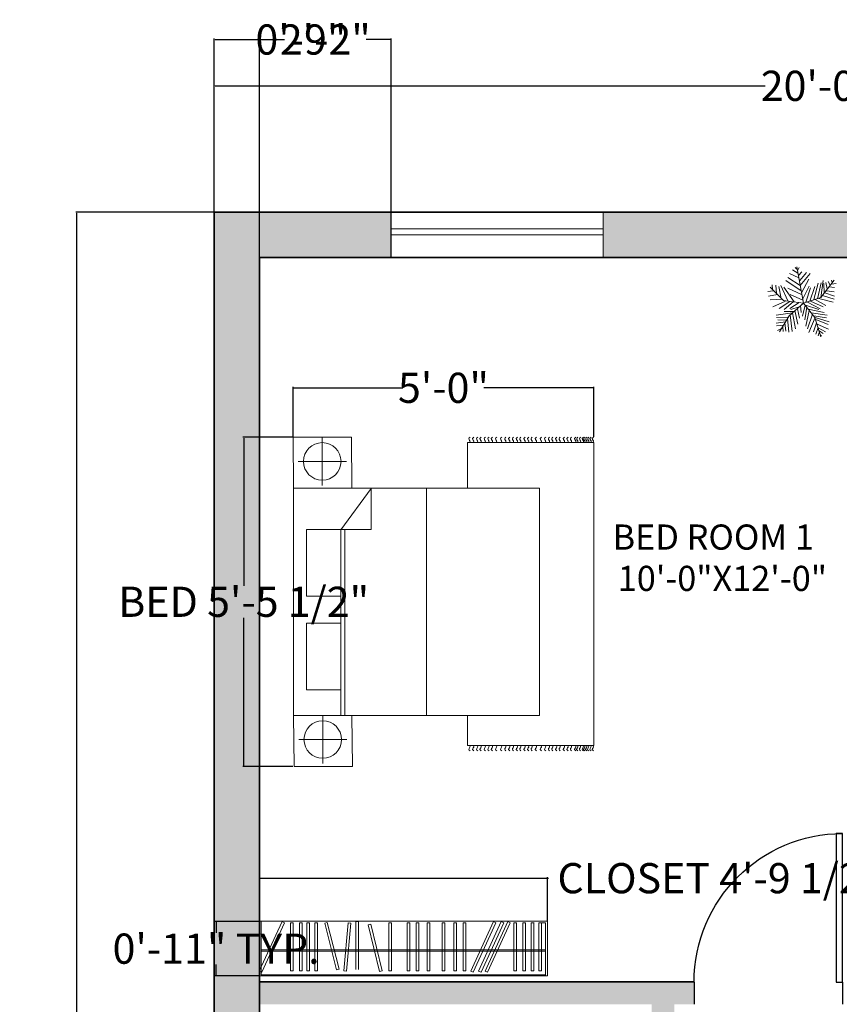
# Model space of a CAD drawing. Units: inches. Extents: x 143233372 to 143233714, y 112671713 to 112672292.
# Tile 6 of 7: x 143233378 to 143233541, y 112672092 to 112672287. Entities that reach past the tile are written whole.
import ezdxf

# ---------------------------------------------------------------- set-up
doc = ezdxf.new("R2010")
doc.units = ezdxf.units.IN
doc.header["$MEASUREMENT"] = 0
doc.layers.get('0').update_dxf_attribs({"color": 104})
for name, color, linetype, lineweight in [('A-ANNO-DIMS', 2, 'Continuous', 18), ('A-AREA-IDEN', 7, 'Continuous', 18), ('closet', 23, 'Continuous', 18), ('doors', 32, 'Continuous', 25), ('furniture', 23, 'Continuous', 18), ('L-PLNT', 92, 'Continuous', 13), ('walls', 7, 'Continuous', 35), ('windows', 4, 'Continuous', 18)]:
    doc.layers.add(name, color=color, linetype=linetype, lineweight=lineweight)
doc.layers.add('A-WALL-PATT', color=18, linetype='Continuous', lineweight=9, true_color=0x000000)
doc.styles.get("Standard").update_dxf_attribs({"font": 'arial.ttf'})
doc.dimstyles.get("Standard").update_dxf_attribs({"dimtxt": 6, "dimasz": 0.18, "dimexe": 0.18, "dimexo": 0.0625, "dimgap": 0.09, "dimtad": 0, "dimtih": 1, "dimtoh": 1, "dimzin": 0, "dimdsep": 46, "dimlunit": 3, "dimtxsty": 'Standard', "dimcen": 0.09, "dimadec": 0, "dimazin": 0, "dimtfac": 1, "dimtofl": 0, "dimtmove": 0, "dimatfit": 3, "dimfxl": 1, "dimtolj": 1, "dimtzin": 0, "dimarcsym": 0})

# ---------------------------------------------------------------- blocks, each defined once
blk = doc.blocks.new('CARPET')
at = {"layer": 'furniture'}
for p, q in [((-51.53, -98.11), (-51.53, -55.12)), ((-51.53, -55.12), (-41.27, -55.12)), ((36, -55.12), (51.55, -55.12)), ((51.55, -55.12), (51.55, -98.11)), ((51.55, -98.11), (-51.53, -98.11))]:
    blk.add_line(p, q, dxfattribs=at)
for points, knots in [([(-53.37, -55.99), (-53.22, -55.8), (-52.9, -55.41), (-52.34, -55.8), (-51.89, -56.08), (-51.65, -55.91), (-51.53, -55.83)], [0, 0, 0, 0, 0.653278, 1.290138, 1.740457, 2.114451, 2.114451, 2.114451, 2.114451]), ([(-53.37, -57.26), (-53.22, -57.07), (-52.9, -56.67), (-52.34, -57.07), (-51.89, -57.35), (-51.65, -57.17), (-51.53, -57.1)], [0, 0, 0, 0, 0.653278, 1.290138, 1.740457, 2.114451, 2.114451, 2.114451, 2.114451]), ([(53.37, -55.99), (53.22, -55.8), (52.9, -55.41), (52.34, -55.8), (51.89, -56.08), (51.65, -55.91), (51.53, -55.83)], [0, 0, 0, 0, 0.653278, 1.290138, 1.740457, 2.114451, 2.114451, 2.114451, 2.114451]), ([(53.37, -57.26), (53.22, -57.07), (52.9, -56.67), (52.34, -57.07), (51.89, -57.35), (51.65, -57.17), (51.53, -57.1)], [0, 0, 0, 0, 0.653278, 1.290138, 1.740457, 2.114451, 2.114451, 2.114451, 2.114451]), ([(-53.37, -58.59), (-53.22, -58.4), (-52.9, -58.01), (-52.34, -58.4), (-51.89, -58.68), (-51.65, -58.5), (-51.53, -58.43)], [0, 0, 0, 0, 0.653278, 1.290138, 1.740457, 2.114451, 2.114451, 2.114451, 2.114451]), ([(-53.37, -59.78), (-53.22, -59.58), (-52.9, -59.19), (-52.34, -59.58), (-51.89, -59.86), (-51.65, -59.69), (-51.53, -59.61)], [0, 0, 0, 0, 0.653278, 1.290138, 1.740457, 2.114451, 2.114451, 2.114451, 2.114451]), ([(53.37, -58.59), (53.22, -58.4), (52.9, -58.01), (52.34, -58.4), (51.89, -58.68), (51.65, -58.5), (51.53, -58.43)], [0, 0, 0, 0, 0.653278, 1.290138, 1.740457, 2.114451, 2.114451, 2.114451, 2.114451]), ([(53.37, -59.78), (53.22, -59.58), (52.9, -59.19), (52.34, -59.58), (51.89, -59.86), (51.65, -59.69), (51.53, -59.61)], [0, 0, 0, 0, 0.653278, 1.290138, 1.740457, 2.114451, 2.114451, 2.114451, 2.114451]), ([(-53.37, -61.22), (-53.22, -61.02), (-52.9, -60.63), (-52.34, -61.02), (-51.89, -61.3), (-51.65, -61.13), (-51.53, -61.05)], [0, 0, 0, 0, 0.653278, 1.290138, 1.740457, 2.114451, 2.114451, 2.114451, 2.114451]), ([(-53.37, -62.44), (-53.22, -62.25), (-52.9, -61.86), (-52.34, -62.25), (-51.89, -62.53), (-51.65, -62.36), (-51.53, -62.28)], [0, 0, 0, 0, 0.653278, 1.290138, 1.740457, 2.114451, 2.114451, 2.114451, 2.114451]), ([(-53.37, -63.63), (-53.22, -63.43), (-52.9, -63.04), (-52.34, -63.43), (-51.89, -63.72), (-51.65, -63.54), (-51.53, -63.46)], [0, 0, 0, 0, 0.653278, 1.290138, 1.740457, 2.114451, 2.114451, 2.114451, 2.114451]), ([(53.37, -61.22), (53.22, -61.02), (52.9, -60.63), (52.34, -61.02), (51.89, -61.3), (51.65, -61.13), (51.53, -61.05)], [0, 0, 0, 0, 0.653278, 1.290138, 1.740457, 2.114451, 2.114451, 2.114451, 2.114451]), ([(53.37, -62.44), (53.22, -62.25), (52.9, -61.86), (52.34, -62.25), (51.89, -62.53), (51.65, -62.36), (51.53, -62.28)], [0, 0, 0, 0, 0.653278, 1.290138, 1.740457, 2.114451, 2.114451, 2.114451, 2.114451]), ([(53.37, -63.63), (53.22, -63.43), (52.9, -63.04), (52.34, -63.43), (51.89, -63.72), (51.65, -63.54), (51.53, -63.46)], [0, 0, 0, 0, 0.653278, 1.290138, 1.740457, 2.114451, 2.114451, 2.114451, 2.114451]), ([(-53.37, -65.07), (-53.22, -64.87), (-52.9, -64.48), (-52.34, -64.87), (-51.89, -65.15), (-51.65, -64.98), (-51.53, -64.9)], [0, 0, 0, 0, 0.653278, 1.290138, 1.740457, 2.114451, 2.114451, 2.114451, 2.114451]), ([(-53.37, -66.76), (-53.22, -66.56), (-52.9, -66.17), (-52.34, -66.56), (-51.89, -66.84), (-51.65, -66.67), (-51.53, -66.59)], [0, 0, 0, 0, 0.653278, 1.290138, 1.740457, 2.114451, 2.114451, 2.114451, 2.114451]), ([(53.37, -65.07), (53.22, -64.87), (52.9, -64.48), (52.34, -64.87), (51.89, -65.15), (51.65, -64.98), (51.53, -64.9)], [0, 0, 0, 0, 0.653278, 1.290138, 1.740457, 2.114451, 2.114451, 2.114451, 2.114451]), ([(53.37, -66.76), (53.22, -66.56), (52.9, -66.17), (52.34, -66.56), (51.89, -66.84), (51.65, -66.67), (51.53, -66.59)], [0, 0, 0, 0, 0.653278, 1.290138, 1.740457, 2.114451, 2.114451, 2.114451, 2.114451]), ([(-53.37, -68.2), (-53.22, -68), (-52.9, -67.61), (-52.34, -68), (-51.89, -68.28), (-51.65, -68.11), (-51.53, -68.03)], [0, 0, 0, 0, 0.653278, 1.290138, 1.740457, 2.114451, 2.114451, 2.114451, 2.114451]), ([(-53.37, -69.53), (-53.22, -69.33), (-52.9, -68.94), (-52.34, -69.33), (-51.89, -69.61), (-51.65, -69.44), (-51.53, -69.36)], [0, 0, 0, 0, 0.653278, 1.290138, 1.740457, 2.114451, 2.114451, 2.114451, 2.114451]), ([(-53.37, -70.79), (-53.22, -70.6), (-52.9, -70.21), (-52.34, -70.6), (-51.89, -70.88), (-51.65, -70.7), (-51.53, -70.63)], [0, 0, 0, 0, 0.653278, 1.290138, 1.740457, 2.114451, 2.114451, 2.114451, 2.114451]), ([(53.37, -68.2), (53.22, -68), (52.9, -67.61), (52.34, -68), (51.89, -68.28), (51.65, -68.11), (51.53, -68.03)], [0, 0, 0, 0, 0.653278, 1.290138, 1.740457, 2.114451, 2.114451, 2.114451, 2.114451]), ([(53.37, -69.53), (53.22, -69.33), (52.9, -68.94), (52.34, -69.33), (51.89, -69.61), (51.65, -69.44), (51.53, -69.36)], [0, 0, 0, 0, 0.653278, 1.290138, 1.740457, 2.114451, 2.114451, 2.114451, 2.114451]), ([(53.37, -70.79), (53.22, -70.6), (52.9, -70.21), (52.34, -70.6), (51.89, -70.88), (51.65, -70.7), (51.53, -70.63)], [0, 0, 0, 0, 0.653278, 1.290138, 1.740457, 2.114451, 2.114451, 2.114451, 2.114451]), ([(-53.37, -72.12), (-53.22, -71.93), (-52.9, -71.54), (-52.34, -71.93), (-51.89, -72.21), (-51.65, -72.04), (-51.53, -71.96)], [0, 0, 0, 0, 0.653278, 1.290138, 1.740457, 2.114451, 2.114451, 2.114451, 2.114451]), ([(-53.37, -73.31), (-53.22, -73.11), (-52.9, -72.72), (-52.34, -73.11), (-51.89, -73.4), (-51.65, -73.22), (-51.53, -73.14)], [0, 0, 0, 0, 0.653278, 1.290138, 1.740457, 2.114451, 2.114451, 2.114451, 2.114451]), ([(53.37, -72.12), (53.22, -71.93), (52.9, -71.54), (52.34, -71.93), (51.89, -72.21), (51.65, -72.04), (51.53, -71.96)], [0, 0, 0, 0, 0.653278, 1.290138, 1.740457, 2.114451, 2.114451, 2.114451, 2.114451]), ([(53.37, -73.31), (53.22, -73.11), (52.9, -72.72), (52.34, -73.11), (51.89, -73.4), (51.65, -73.22), (51.53, -73.14)], [0, 0, 0, 0, 0.653278, 1.290138, 1.740457, 2.114451, 2.114451, 2.114451, 2.114451]), ([(-53.37, -74.75), (-53.22, -74.55), (-52.9, -74.16), (-52.34, -74.55), (-51.89, -74.83), (-51.65, -74.66), (-51.53, -74.58)], [0, 0, 0, 0, 0.653278, 1.290138, 1.740457, 2.114451, 2.114451, 2.114451, 2.114451]), ([(-53.37, -75.98), (-53.22, -75.78), (-52.9, -75.39), (-52.34, -75.78), (-51.89, -76.06), (-51.65, -75.89), (-51.53, -75.81)], [0, 0, 0, 0, 0.653278, 1.290138, 1.740457, 2.114451, 2.114451, 2.114451, 2.114451]), ([(-53.37, -77.16), (-53.22, -76.96), (-52.9, -76.57), (-52.34, -76.96), (-51.89, -77.25), (-51.65, -77.07), (-51.53, -76.99)], [0, 0, 0, 0, 0.653278, 1.290138, 1.740457, 2.114451, 2.114451, 2.114451, 2.114451]), ([(53.37, -74.75), (53.22, -74.55), (52.9, -74.16), (52.34, -74.55), (51.89, -74.83), (51.65, -74.66), (51.53, -74.58)], [0, 0, 0, 0, 0.653278, 1.290138, 1.740457, 2.114451, 2.114451, 2.114451, 2.114451]), ([(53.37, -75.98), (53.22, -75.78), (52.9, -75.39), (52.34, -75.78), (51.89, -76.06), (51.65, -75.89), (51.53, -75.81)], [0, 0, 0, 0, 0.653278, 1.290138, 1.740457, 2.114451, 2.114451, 2.114451, 2.114451]), ([(53.37, -77.16), (53.22, -76.96), (52.9, -76.57), (52.34, -76.96), (51.89, -77.25), (51.65, -77.07), (51.53, -76.99)], [0, 0, 0, 0, 0.653278, 1.290138, 1.740457, 2.114451, 2.114451, 2.114451, 2.114451]), ([(-53.37, -78.6), (-53.22, -78.4), (-52.9, -78.01), (-52.34, -78.4), (-51.89, -78.68), (-51.65, -78.51), (-51.53, -78.43)], [0, 0, 0, 0, 0.653278, 1.290138, 1.740457, 2.114451, 2.114451, 2.114451, 2.114451]), ([(-53.37, -80.29), (-53.22, -80.09), (-52.9, -79.7), (-52.34, -80.09), (-51.89, -80.37), (-51.65, -80.2), (-51.53, -80.12)], [0, 0, 0, 0, 0.653278, 1.290138, 1.740457, 2.114451, 2.114451, 2.114451, 2.114451]), ([(53.37, -78.6), (53.22, -78.4), (52.9, -78.01), (52.34, -78.4), (51.89, -78.68), (51.65, -78.51), (51.53, -78.43)], [0, 0, 0, 0, 0.653278, 1.290138, 1.740457, 2.114451, 2.114451, 2.114451, 2.114451]), ([(53.37, -80.29), (53.22, -80.09), (52.9, -79.7), (52.34, -80.09), (51.89, -80.37), (51.65, -80.2), (51.53, -80.12)], [0, 0, 0, 0, 0.653278, 1.290138, 1.740457, 2.114451, 2.114451, 2.114451, 2.114451]), ([(-53.37, -81.73), (-53.22, -81.53), (-52.9, -81.14), (-52.34, -81.53), (-51.89, -81.81), (-51.65, -81.64), (-51.53, -81.56)], [0, 0, 0, 0, 0.653278, 1.290138, 1.740457, 2.114451, 2.114451, 2.114451, 2.114451]), ([(-53.37, -83.06), (-53.22, -82.86), (-52.9, -82.47), (-52.34, -82.86), (-51.89, -83.14), (-51.65, -82.97), (-51.53, -82.89)], [0, 0, 0, 0, 0.653278, 1.290138, 1.740457, 2.114451, 2.114451, 2.114451, 2.114451]), ([(-53.37, -84.18), (-53.22, -83.99), (-52.9, -83.6), (-52.34, -83.99), (-51.89, -84.27), (-51.65, -84.09), (-51.53, -84.02)], [0, 0, 0, 0, 0.653278, 1.290138, 1.740457, 2.114451, 2.114451, 2.114451, 2.114451]), ([(53.37, -81.73), (53.22, -81.53), (52.9, -81.14), (52.34, -81.53), (51.89, -81.81), (51.65, -81.64), (51.53, -81.56)], [0, 0, 0, 0, 0.653278, 1.290138, 1.740457, 2.114451, 2.114451, 2.114451, 2.114451]), ([(53.37, -83.06), (53.22, -82.86), (52.9, -82.47), (52.34, -82.86), (51.89, -83.14), (51.65, -82.97), (51.53, -82.89)], [0, 0, 0, 0, 0.653278, 1.290138, 1.740457, 2.114451, 2.114451, 2.114451, 2.114451]), ([(53.37, -84.18), (53.22, -83.99), (52.9, -83.6), (52.34, -83.99), (51.89, -84.27), (51.65, -84.09), (51.53, -84.02)], [0, 0, 0, 0, 0.653278, 1.290138, 1.740457, 2.114451, 2.114451, 2.114451, 2.114451]), ([(-53.37, -85.51), (-53.22, -85.32), (-52.9, -84.93), (-52.34, -85.32), (-51.89, -85.6), (-51.65, -85.42), (-51.53, -85.35)], [0, 0, 0, 0, 0.653278, 1.290138, 1.740457, 2.114451, 2.114451, 2.114451, 2.114451]), ([(-53.37, -86.7), (-53.22, -86.5), (-52.9, -86.11), (-52.34, -86.5), (-51.89, -86.78), (-51.65, -86.61), (-51.53, -86.53)], [0, 0, 0, 0, 0.653278, 1.290138, 1.740457, 2.114451, 2.114451, 2.114451, 2.114451]), ([(53.37, -85.51), (53.22, -85.32), (52.9, -84.93), (52.34, -85.32), (51.89, -85.6), (51.65, -85.42), (51.53, -85.35)], [0, 0, 0, 0, 0.653278, 1.290138, 1.740457, 2.114451, 2.114451, 2.114451, 2.114451]), ([(53.37, -86.7), (53.22, -86.5), (52.9, -86.11), (52.34, -86.5), (51.89, -86.78), (51.65, -86.61), (51.53, -86.53)], [0, 0, 0, 0, 0.653278, 1.290138, 1.740457, 2.114451, 2.114451, 2.114451, 2.114451]), ([(-53.37, -88.14), (-53.22, -87.94), (-52.9, -87.55), (-52.34, -87.94), (-51.89, -88.22), (-51.65, -88.05), (-51.53, -87.97)], [0, 0, 0, 0, 0.653278, 1.290138, 1.740457, 2.114451, 2.114451, 2.114451, 2.114451]), ([(-53.37, -89.36), (-53.22, -89.17), (-52.9, -88.78), (-52.34, -89.17), (-51.89, -89.45), (-51.65, -89.28), (-51.53, -89.2)], [0, 0, 0, 0, 0.653278, 1.290138, 1.740457, 2.114451, 2.114451, 2.114451, 2.114451]), ([(-53.37, -90.55), (-53.22, -90.35), (-52.9, -89.96), (-52.34, -90.35), (-51.89, -90.64), (-51.65, -90.46), (-51.53, -90.38)], [0, 0, 0, 0, 0.653278, 1.290138, 1.740457, 2.114451, 2.114451, 2.114451, 2.114451]), ([(53.37, -88.14), (53.22, -87.94), (52.9, -87.55), (52.34, -87.94), (51.89, -88.22), (51.65, -88.05), (51.53, -87.97)], [0, 0, 0, 0, 0.653278, 1.290138, 1.740457, 2.114451, 2.114451, 2.114451, 2.114451]), ([(53.37, -89.36), (53.22, -89.17), (52.9, -88.78), (52.34, -89.17), (51.89, -89.45), (51.65, -89.28), (51.53, -89.2)], [0, 0, 0, 0, 0.653278, 1.290138, 1.740457, 2.114451, 2.114451, 2.114451, 2.114451]), ([(53.37, -90.55), (53.22, -90.35), (52.9, -89.96), (52.34, -90.35), (51.9, -90.63), (51.66, -90.47), (51.55, -90.4)], [0, 0, 0, 0, 0.653278, 1.290138, 1.740457, 2.0926, 2.0926, 2.0926, 2.0926]), ([(-53.37, -91.99), (-53.22, -91.79), (-52.9, -91.4), (-52.34, -91.79), (-51.89, -92.07), (-51.65, -91.9), (-51.53, -91.82)], [0, 0, 0, 0, 0.653278, 1.290138, 1.740457, 2.114451, 2.114451, 2.114451, 2.114451]), ([(-53.37, -92.69), (-53.22, -92.48), (-52.9, -92.08), (-52.35, -92.49), (-51.89, -92.77), (-51.65, -92.6), (-51.53, -92.52)], [0, 0, 0, 0, 0.663904, 1.307406, 1.757725, 2.131719, 2.131719, 2.131719, 2.131719]), ([(-53.37, -93.61), (-53.22, -93.42), (-52.9, -93.03), (-52.34, -93.42), (-51.89, -93.7), (-51.65, -93.52), (-51.53, -93.45)], [0, 0, 0, 0, 0.653278, 1.290138, 1.740457, 2.114451, 2.114451, 2.114451, 2.114451]), ([(53.37, -91.99), (53.22, -91.79), (52.9, -91.4), (52.34, -91.79), (51.9, -92.07), (51.66, -91.91), (51.55, -91.83)], [0, 0, 0, 0, 0.653278, 1.290138, 1.740457, 2.0926, 2.0926, 2.0926, 2.0926]), ([(53.37, -92.69), (53.22, -92.49), (52.9, -92.09), (52.34, -92.49), (51.9, -92.77), (51.66, -92.61), (51.55, -92.53)], [0, 0, 0, 0, 0.656792, 1.295826, 1.746145, 2.098292, 2.098292, 2.098292, 2.098292]), ([(53.37, -93.66), (53.22, -93.46), (52.9, -93.07), (52.34, -93.46), (51.9, -93.74), (51.66, -93.58), (51.55, -93.5)], [0, 0, 0, 0, 0.653278, 1.290138, 1.740457, 2.0926, 2.0926, 2.0926, 2.0926]), ([(-53.37, -94.55), (-53.22, -94.35), (-52.9, -93.96), (-52.34, -94.35), (-51.89, -94.63), (-51.65, -94.46), (-51.53, -94.38)], [0, 0, 0, 0, 0.653278, 1.290138, 1.740457, 2.114451, 2.114451, 2.114451, 2.114451]), ([(-53.37, -95.05), (-53.22, -94.85), (-52.9, -94.46), (-52.34, -94.85), (-51.89, -95.14), (-51.65, -94.96), (-51.53, -94.88)], [0, 0, 0, 0, 0.653278, 1.290138, 1.740457, 2.114451, 2.114451, 2.114451, 2.114451]), ([(-53.37, -95.73), (-53.22, -95.54), (-52.9, -95.15), (-52.34, -95.54), (-51.89, -95.82), (-51.65, -95.65), (-51.53, -95.57)], [0, 0, 0, 0, 0.653278, 1.290138, 1.740457, 2.114451, 2.114451, 2.114451, 2.114451]), ([(-53.37, -96.38), (-53.22, -96.18), (-52.9, -95.79), (-52.34, -96.18), (-51.89, -96.47), (-51.65, -96.29), (-51.53, -96.21)], [0, 0, 0, 0, 0.653278, 1.290138, 1.740457, 2.114451, 2.114451, 2.114451, 2.114451]), ([(-53.37, -97.17), (-53.22, -96.98), (-52.9, -96.59), (-52.34, -96.98), (-51.89, -97.26), (-51.65, -97.08), (-51.53, -97.01)], [0, 0, 0, 0, 0.653278, 1.290138, 1.740457, 2.114451, 2.114451, 2.114451, 2.114451]), ([(53.37, -95.78), (53.22, -95.58), (52.9, -95.19), (52.34, -95.58), (51.89, -95.86), (51.65, -95.69), (51.53, -95.61)], [0, 0, 0, 0, 0.653278, 1.290138, 1.740457, 2.114451, 2.114451, 2.114451, 2.114451]), ([(53.37, -96.43), (53.22, -96.23), (52.9, -95.84), (52.34, -96.23), (51.89, -96.51), (51.65, -96.34), (51.53, -96.26)], [0, 0, 0, 0, 0.653278, 1.290138, 1.740457, 2.114451, 2.114451, 2.114451, 2.114451]), ([(53.37, -97.22), (53.22, -97.02), (52.9, -96.63), (52.34, -97.02), (51.89, -97.3), (51.65, -97.13), (51.53, -97.05)], [0, 0, 0, 0, 0.653278, 1.290138, 1.740457, 2.114451, 2.114451, 2.114451, 2.114451]), ([(53.37, -94.59), (53.22, -94.4), (52.9, -94.01), (52.34, -94.4), (51.9, -94.68), (51.66, -94.51), (51.55, -94.44)], [0, 0, 0, 0, 0.653278, 1.290138, 1.740457, 2.0926, 2.0926, 2.0926, 2.0926]), ([(53.37, -95.1), (53.22, -94.9), (52.9, -94.51), (52.34, -94.9), (51.9, -95.18), (51.66, -95.02), (51.55, -94.94)], [0, 0, 0, 0, 0.653278, 1.290138, 1.740457, 2.0926, 2.0926, 2.0926, 2.0926]), ([(-53.37, -97.99), (-53.22, -97.79), (-52.9, -97.4), (-52.34, -97.79), (-51.89, -98.08), (-51.65, -97.9), (-51.53, -97.82)], [0, 0, 0, 0, 0.653278, 1.290138, 1.740457, 2.114451, 2.114451, 2.114451, 2.114451]), ([(53.37, -97.99), (53.22, -97.79), (52.9, -97.4), (52.34, -97.79), (51.89, -98.08), (51.65, -97.9), (51.53, -97.82)], [0, 0, 0, 0, 0.653278, 1.290138, 1.740457, 2.114451, 2.114451, 2.114451, 2.114451])]:
    blk.add_open_spline(points, degree=3, knots=knots, dxfattribs=at)
blk = doc.blocks.new('A$C58D270C6')
at = {"layer": 'furniture'}
for p, q in [((9.09, 124.13), (9.09, 108.87)), ((1.46, 116.5), (16.73, 116.5)), ((14.97, 94.84), (24.62, 107.92)), ((24.62, 94.93), (24.62, 107.92)), ((42.08, 108), (42.08, 36)), ((14.97, 94.93), (24.62, 94.93)), ((14.97, 94.84), (14.97, 36)), ((16.22, 94.93), (16.22, 36)), ((9.25, 36), (9.25, 20.74)), ((1.62, 28.37), (16.88, 28.37))]:
    blk.add_line(p, q, dxfattribs=at)
for points in [[(18.5, 108), (18.34, 124.13), (-0.16, 124.13), (0, 108)], [(0, 108), (77.91, 108), (77.91, 36), (0, 36)], [(4.09, 94.93), (14.97, 94.93), (14.97, 73.83), (4.09, 73.83)], [(4.09, 65.23), (14.97, 65.23), (14.97, 44.13), (4.09, 44.13)], [(18.65, 19.87), (18.5, 36), (0, 36), (0.16, 19.87)]]:
    blk.add_lwpolyline(points, close=True, dxfattribs=at)
for centre in [(9.09, 116.5), (9.25, 28.37)]:
    blk.add_circle(centre, 5.95, dxfattribs=at)
at = {"layer": 'furniture', "xscale": 0.9312884925094044, "yscale": 0.9312884925094044, "zscale": 0.9312884925094044, "rotation": 90}
blk.add_blockref('CARPET', (3.79, 74.47), dxfattribs=at)
blk = doc.blocks.new('closet')
at = {"layer": 'closet'}
for p, q in [((26.09, 8.25), (26.09, -5.1)), ((26.84, 8.25), (26.84, -5.1)), ((-0.71, -5.58), (5.59, 8.19)), ((-0.23, 7.39), (-0.23, -6.57)), ((6.27, 7.88), (-0.04, -5.89)), ((5.59, 8.19), (6.27, 7.88)), ((7.92, 7.84), (8.68, 7.84)), ((7.92, 7.84), (7.92, -5.51)), ((8.68, 7.84), (8.68, -5.51)), ((10.44, 7.84), (11.2, 7.84)), ((10.44, 7.84), (10.44, -5.51)), ((11.2, 7.84), (11.2, -5.51)), ((12.45, 7.84), (13.21, 7.84)), ((12.45, 7.84), (12.45, -5.51)), ((13.21, 7.84), (13.21, -5.51)), ((14.71, 7.84), (15.47, 7.84)), ((14.71, 7.84), (14.71, -5.51)), ((15.47, 7.84), (15.47, -5.51)), ((17.44, 7.75), (18.17, 7.93)), ((17.44, 7.75), (20.73, -5.2)), ((18.17, 7.93), (21.46, -5.01)), ((23.92, 7.84), (22.75, -5.46)), ((24.67, 7.78), (23.51, -5.53)), ((23.92, 7.84), (24.67, 7.78)), ((29.49, 7.29), (32.64, -5.69)), ((30.22, 7.46), (33.37, -5.51)), ((35.23, 7.84), (35.23, -5.51)), ((35.99, 7.84), (35.99, -5.51)), ((40.33, 7.84), (40.33, -5.51)), ((41.08, 7.84), (41.08, -5.51)), ((42.85, 7.84), (42.85, -5.51)), ((43.61, 7.84), (43.61, -5.51)), ((45.9, 7.84), (45.9, -5.51)), ((46.65, 7.84), (46.65, -5.51)), ((50.07, 7.84), (50.07, -5.51)), ((50.82, 7.84), (50.82, -5.51)), ((53.32, 7.84), (53.32, -5.51)), ((54.08, 7.84), (54.08, -5.51)), ((55.9, 7.84), (55.9, -5.51)), ((56.65, 7.84), (56.65, -5.51)), ((57.99, -5.58), (64.3, 8.19)), ((64.97, 7.88), (58.67, -5.89)), ((60.19, -5.58), (66.49, 8.19)), ((67.17, 7.88), (60.87, -5.89)), ((62, -5.58), (68.3, 8.19)), ((68.98, 7.88), (62.67, -5.89)), ((69.96, 7.84), (69.96, -5.51)), ((70.72, 7.84), (70.72, -5.51)), ((72.43, 7.84), (72.43, -5.51)), ((73.19, 7.84), (73.19, -5.51)), ((74.82, 7.84), (74.82, -5.51)), ((75.57, 7.84), (75.57, -5.51)), ((76.94, 7.84), (76.94, -5.51)), ((77.69, 7.84), (77.69, -5.51)), ((56.23, 0.33), (0, 0.33)), ((56.2, 0), (0, 0)), ((56.2, 0), (78.76, 0)), ((56.23, 0.33), (78.76, 0.33)), ((21.46, -5.01), (20.73, -5.2)), ((23.51, -5.53), (22.75, -5.46)), ((-0.04, -5.89), (-0.71, -5.58)), ((33.37, -5.51), (32.64, -5.69)), ((35.99, -5.51), (35.23, -5.51)), ((41.08, -5.51), (40.33, -5.51)), ((43.61, -5.51), (42.85, -5.51)), ((46.65, -5.51), (45.9, -5.51)), ((50.82, -5.51), (50.07, -5.51)), ((54.08, -5.51), (53.32, -5.51)), ((56.65, -5.51), (55.9, -5.51)), ((58.67, -5.89), (57.99, -5.58)), ((60.87, -5.89), (60.19, -5.58)), ((62.67, -5.89), (62, -5.58)), ((70.72, -5.51), (69.96, -5.51)), ((73.19, -5.51), (72.43, -5.51)), ((75.57, -5.51), (74.82, -5.51)), ((77.69, -5.51), (76.94, -5.51))]:
    blk.add_line(p, q, dxfattribs=at)
blk = doc.blocks.new('rotated closet')
at = {"layer": 'closet'}
for p, q in [((26.32, 0.86), (27.07, 0.86)), ((29.72, -0.11), (30.45, 0.07)), ((35.46, 0.45), (36.22, 0.45)), ((40.56, 0.45), (41.31, 0.45)), ((43.08, 0.45), (43.84, 0.45)), ((46.13, 0.45), (46.88, 0.45)), ((50.3, 0.45), (51.05, 0.45)), ((53.56, 0.45), (54.31, 0.45)), ((56.13, 0.45), (56.88, 0.45)), ((64.53, 0.8), (65.2, 0.49)), ((66.72, 0.8), (67.4, 0.49)), ((68.53, 0.8), (69.21, 0.49)), ((70.19, 0.45), (70.95, 0.45)), ((72.66, 0.45), (73.42, 0.45)), ((75.05, 0.45), (75.81, 0.45)), ((77.17, 0.45), (77.92, 0.45)), ((78.99, 0), (78.99, -13.96)), ((8.91, -12.91), (8.15, -12.91)), ((11.43, -12.91), (10.67, -12.91)), ((13.44, -12.91), (12.68, -12.91)), ((15.7, -12.91), (14.94, -12.91)), ((-0.46, -14.27), (79.54, -14.27)), ((0, -13.96), (78.99, -13.96))]:
    blk.add_line(p, q, dxfattribs=at)
blk.add_blockref('closet', (0.23, -7.39), dxfattribs=at)
blk = doc.blocks.new('*U24')
for p, q in [((0, 0), (0, -6)), ((40, 0), (40, -6))]:
    blk.add_line(p, q)
blk.add_lwpolyline([(0, 0), (0, 40), (1.75, 40), (1.75, 0)], close=True)
blk.add_arc((0, 0), 40, 0, 90)
blk = doc.blocks.new('*U26')
for p, q in [((-7.288, 39.707), (-21.778, 46.673)), ((-8.737, 47.138), (-17.069, 52.711)), ((-10.186, 53.64), (-13.084, 55.962)), ((0, 0), (-10.5, 57)), ((-9.099, 51.782), (-6.563, 55.962)), ((-7.65, 43.423), (-2.578, 49.46)), ((-5.839, 35.992), (4.667, 48.067)), ((-5.114, 27.632), (10.463, 46.673)), ((-3.665, 19.273), (-27.574, 35.527)), ((-5.114, 28.097), (-24.676, 40.636)), ((-2.941, 16.486), (8.652, 37.85)), ((16.259, 5.805), (23.142, 31.348)), ((22.055, 7.198), (27.489, 32.277)), ((27, 9), (48, 36)), ((27.127, 9.056), (31.112, 35.992)), ((35.096, 32.741), (37.27, 22.524)), ((38.719, 34.134), (41.979, 28.561)), ((44.153, 36.456), (45.239, 32.741)), ((-47.498, 19.737), (-55.83, 18.344)), ((-31.5, 4.5), (-52.5, 25.5)), ((-48.585, 21.131), (-49.309, 29.026)), ((-43.513, 28.561), (-42.427, 15.558)), ((-38.442, 26.239), (-34.819, 7.663)), ((-35.544, 28.097), (-24.314, 3.947)), ((-14.533, 2.09), (-30.834, 25.31)), ((-24.314, 23.917), (-2.941, 13.7)), ((-1.129, 6.734), (9.014, 26.704)), ((3.942, 1.625), (11.187, 24.381)), ((10.101, 3.483), (17.708, 26.239)), ((31.836, 30.883), (32.561, 16.486)), ((33.285, 16.486), (48.862, 10.913)), ((36.183, 19.737), (48.137, 17.88)), ((40.53, 25.775), (48.862, 24.846)), ((43.791, 29.954), (51.036, 30.883)), ((-40.615, 13.7), (-55.105, 10.913)), ((-33.37, 6.269), (-52.207, 5.34)), ((-28.299, 3.483), (-47.86, -5.805)), ((-21.416, 3.018), (-38.079, -8.128)), ((0, 0), (-31.5, 4.5)), ((-15.982, 2.09), (-30.11, -9.521)), ((0, 0), (-22.5, -19.5)), ((-6.563, 1.161), (-21.416, -8.128)), ((-20.691, 13.7), (-1.129, 4.876)), ((0, 0), (27, 9)), ((0, 0), (18, -22.5)), ((6.478, 1.625), (26.04, -8.592)), ((11.187, 3.483), (30.749, -5.805)), ((18.07, 5.805), (35.096, -3.483)), ((24.229, 7.663), (46.688, 1.625)), ((29.662, 12.307), (48.137, 6.269)), ((-17.431, -15.094), (-42.789, -18.809)), ((-15.257, -12.772), (-30.11, -12.772)), ((-6.563, -5.805), (-19.967, -9.985)), ((-17.069, -15.094), (-12.721, -40.172)), ((-13.446, -11.378), (-8.737, -32.741)), ((-9.461, -8.592), (-6.201, -23.453)), ((-4.752, -3.483), (-3.665, -14.629)), ((2.493, -3.019), (-1.491, -20.202)), ((1.769, -2.555), (24.229, -9.521)), ((5.029, -6.27), (2.131, -25.775)), ((9.014, -11.378), (3.58, -35.992)), ((7.565, -9.056), (32.198, -14.629)), ((12.274, -15.094), (36.907, -18.809)), ((-28.299, -29.026), (-42.789, -31.348)), ((-24.314, -21.596), (-42.427, -22.06)), ((-26.849, -26.24), (-40.253, -25.775)), ((-22.5, -19.5), (-37.5, -45)), ((-29.023, -30.884), (-27.936, -43.887)), ((-25.038, -23.918), (-22.865, -45.281)), ((-20.691, -18.345), (-17.793, -44.352)), ((14.085, -16.951), (6.478, -40.172)), ((18.07, -22.524), (8.289, -45.745)), ((20.244, -30.419), (15.897, -44.816)), ((16.259, -19.738), (36.183, -22.989)), ((18, -22.5), (27, -52.5)), ((18.433, -22.524), (40.53, -29.026)), ((19.157, -25.311), (38.719, -33.206)), ((-30.834, -34.135), (-42.427, -35.528)), ((-34.457, -39.708), (-40.978, -42.494)), ((-32.646, -36.921), (-31.921, -44.352)), ((22.78, -37.85), (19.519, -48.532)), ((21.331, -32.741), (39.081, -40.636)), ((22.78, -38.314), (34.372, -44.816)), ((24.591, -45.745), (23.142, -50.854)), ((24.591, -43.423), (30.749, -47.603)), ((26.764, -49.925), (28.213, -50.854))]:
    blk.add_line(p, q)
blk = doc.blocks.new('*D27')
at = {"layer": 'A-ANNO-DIMS', "color": 0, "lineweight": -2, "transparency": 16777216}
for p, q in [((143233416.28, 112672249.24), (143233416.28, 112672274.49)), ((143233416.46, 112672274.31), (143233525.84, 112672274.31)), ((143233656.1, 112672274.31), (143233546.73, 112672274.31)), ((143233656.28, 112672249.24), (143233656.28, 112672274.49))]:
    blk.add_line(p, q, dxfattribs=at)
at = {"layer": 'A-ANNO-DIMS', "color": 0, "transparency": 16777216}
for points in [[(143233416.46, 112672274.34), (143233416.46, 112672274.28), (143233416.28, 112672274.31)], [(143233656.1, 112672274.34), (143233656.1, 112672274.28), (143233656.28, 112672274.31)]]:
    blk.add_solid(points, dxfattribs=at)
at = {"layer": 'Defpoints', "color": 0, "transparency": 16777216}
for p in [(143233656.28, 112672274.31), (143233416.28, 112672249.18), (143233656.28, 112672249.18)]:
    blk.add_point(p, dxfattribs=at)
at = {"layer": 'A-ANNO-DIMS', "color": 0, "transparency": 16777216, "insert": (143233536.28, 112672274.31), "char_height": 6, "attachment_point": 5}
blk.add_mtext('\\A1;20\'-0"', dxfattribs=at)
blk = doc.blocks.new('*D28')
at = {"layer": 'A-ANNO-DIMS', "color": 0, "lineweight": -2, "transparency": 16777216}
for p, q in [((143233416.22, 112672249.18), (143233388.75, 112672249.18)), ((143233388.93, 112672249), (143233388.93, 112672011.59)), ((143233388.93, 112671767.86), (143233388.93, 112672005.28)), ((143233416.22, 112671767.68), (143233388.75, 112671767.68))]:
    blk.add_line(p, q, dxfattribs=at)
at = {"layer": 'A-ANNO-DIMS', "color": 0, "transparency": 16777216}
for points in [[(143233388.9, 112672249), (143233388.96, 112672249), (143233388.93, 112672249.18)], [(143233388.9, 112671767.86), (143233388.96, 112671767.86), (143233388.93, 112671767.68)]]:
    blk.add_solid(points, dxfattribs=at)
at = {"layer": 'Defpoints', "color": 0, "transparency": 16777216}
for p in [(143233416.28, 112672249.18), (143233388.93, 112671767.68), (143233416.28, 112671767.68)]:
    blk.add_point(p, dxfattribs=at)
at = {"layer": 'A-ANNO-DIMS', "color": 0, "transparency": 16777216, "insert": (143233388.93, 112672008.43), "char_height": 6, "attachment_point": 5}
blk.add_mtext('\\A1;30\'-0"', dxfattribs=at)
blk = doc.blocks.new('SASH-42IN')
for p, q in [((0, 1.17), (42.12, 1.17)), ((42.12, 0), (0, 0)), ((42.12, 1.17), (42.12, 0))]:
    blk.add_line(p, q)
blk = doc.blocks.new('*D41')
at = {"layer": 'A-ANNO-DIMS', "color": 0, "lineweight": -2, "transparency": 16777216}
for p, q in [((143233431.91, 112672204.45), (143233421.98, 112672204.45)), ((143233422.16, 112672204.27), (143233422.16, 112672174.92)), ((143233422.16, 112672139.18), (143233422.16, 112672168.53)), ((143233431.91, 112672139), (143233421.98, 112672139))]:
    blk.add_line(p, q, dxfattribs=at)
at = {"layer": 'A-ANNO-DIMS', "color": 0, "transparency": 16777216}
for points in [[(143233422.13, 112672204.27), (143233422.19, 112672204.27), (143233422.16, 112672204.45)], [(143233422.13, 112672139.18), (143233422.19, 112672139.18), (143233422.16, 112672139)]]:
    blk.add_solid(points, dxfattribs=at)
at = {"layer": 'Defpoints', "color": 0, "transparency": 16777216}
for p in [(143233422.16, 112672204.45), (143233431.98, 112672204.45), (143233431.98, 112672139)]:
    blk.add_point(p, dxfattribs=at)
at = {"layer": 'A-ANNO-DIMS', "color": 0, "transparency": 16777216, "insert": (143233422.16, 112672171.72), "char_height": 6, "attachment_point": 5}
blk.add_mtext('\\A1;BED 5\'-5 1/2"', dxfattribs=at)
blk = doc.blocks.new('*D42')
at = {"layer": 'A-ANNO-DIMS', "color": 0, "lineweight": -2, "transparency": 16777216}
for p, q in [((143233431.98, 112672204.51), (143233431.98, 112672214.45)), ((143233432.16, 112672214.27), (143233453.82, 112672214.27)), ((143233491.6, 112672214.27), (143233469.94, 112672214.27)), ((143233491.78, 112672204.51), (143233491.78, 112672214.45))]:
    blk.add_line(p, q, dxfattribs=at)
at = {"layer": 'A-ANNO-DIMS', "color": 0, "transparency": 16777216}
for points in [[(143233432.16, 112672214.3), (143233432.16, 112672214.24), (143233431.98, 112672214.27)], [(143233491.6, 112672214.3), (143233491.6, 112672214.24), (143233491.78, 112672214.27)]]:
    blk.add_solid(points, dxfattribs=at)
at = {"layer": 'Defpoints', "color": 0, "transparency": 16777216}
for p in [(143233491.78, 112672214.27), (143233431.98, 112672204.45), (143233491.78, 112672204.45)]:
    blk.add_point(p, dxfattribs=at)
at = {"layer": 'A-ANNO-DIMS', "color": 0, "transparency": 16777216, "insert": (143233461.88, 112672214.27), "char_height": 6, "attachment_point": 5}
blk.add_mtext('\\A1;5\'-0"', dxfattribs=at)
blk = doc.blocks.new('*D47')
at = {"layer": 'A-ANNO-DIMS', "color": 0, "lineweight": -2, "transparency": 16777216}
for p, q in [((143233425.27, 112672108.23), (143233425.27, 112672116.94)), ((143233425.45, 112672116.76), (143233482.38, 112672116.76)), ((143233482.56, 112672108.23), (143233482.56, 112672116.94)), ((143233482.56, 112672116.76), (143233482.74, 112672116.76))]:
    blk.add_line(p, q, dxfattribs=at)
at = {"layer": 'A-ANNO-DIMS', "color": 0, "transparency": 16777216}
for points in [[(143233425.45, 112672116.79), (143233425.45, 112672116.73), (143233425.27, 112672116.76)], [(143233482.38, 112672116.79), (143233482.38, 112672116.73), (143233482.56, 112672116.76)]]:
    blk.add_solid(points, dxfattribs=at)
at = {"layer": 'Defpoints', "color": 0, "transparency": 16777216}
for p in [(143233482.56, 112672116.76), (143233425.27, 112672108.17), (143233482.56, 112672108.17)]:
    blk.add_point(p, dxfattribs=at)
at = {"layer": 'A-ANNO-DIMS', "color": 0, "transparency": 16777216, "insert": (143233526.01, 112672116.76), "char_height": 6, "attachment_point": 5}
blk.add_mtext('\\A1;CLOSET 4\'-9 1/2" TYP.', dxfattribs=at)
blk = doc.blocks.new('*D48')
at = {"layer": 'A-ANNO-DIMS', "color": 0, "lineweight": -2, "transparency": 16777216}
for p, q in [((143233425.21, 112672108.17), (143233416.49, 112672108.17)), ((143233416.67, 112672107.99), (143233416.67, 112672105.9)), ((143233416.67, 112672097.51), (143233416.67, 112672099.6)), ((143233425.21, 112672097.33), (143233416.49, 112672097.33))]:
    blk.add_line(p, q, dxfattribs=at)
at = {"layer": 'A-ANNO-DIMS', "color": 0, "transparency": 16777216}
for points in [[(143233416.64, 112672107.99), (143233416.7, 112672107.99), (143233416.67, 112672108.17)], [(143233416.64, 112672097.51), (143233416.7, 112672097.51), (143233416.67, 112672097.33)]]:
    blk.add_solid(points, dxfattribs=at)
at = {"layer": 'Defpoints', "color": 0, "transparency": 16777216}
for p in [(143233416.67, 112672108.17), (143233425.27, 112672108.17), (143233425.27, 112672097.33)]:
    blk.add_point(p, dxfattribs=at)
at = {"layer": 'A-ANNO-DIMS', "color": 0, "transparency": 16777216, "insert": (143233416.67, 112672102.75), "char_height": 6, "attachment_point": 5}
blk.add_mtext('\\A1;0\'-11" TYP.', dxfattribs=at)
blk = doc.blocks.new('*D64')
at = {"layer": 'A-ANNO-DIMS', "color": 0, "lineweight": -2, "transparency": 16777216}
for p, q in [((143233416.28, 112672249.24), (143233416.28, 112672283.7)), ((143233416.46, 112672283.52), (143233425.1, 112672283.52)), ((143233425.28, 112672240.24), (143233425.28, 112672283.7)), ((143233425.28, 112672283.52), (143233425.46, 112672283.52))]:
    blk.add_line(p, q, dxfattribs=at)
at = {"layer": 'A-ANNO-DIMS', "color": 0, "transparency": 16777216}
for points in [[(143233416.46, 112672283.55), (143233416.46, 112672283.49), (143233416.28, 112672283.52)], [(143233425.1, 112672283.55), (143233425.1, 112672283.49), (143233425.28, 112672283.52)]]:
    blk.add_solid(points, dxfattribs=at)
at = {"layer": 'Defpoints', "color": 0, "transparency": 16777216}
for p in [(143233425.28, 112672283.52), (143233416.28, 112672249.18), (143233425.28, 112672240.18)]:
    blk.add_point(p, dxfattribs=at)
at = {"layer": 'A-ANNO-DIMS', "color": 0, "transparency": 16777216, "insert": (143233433.53, 112672283.52), "char_height": 6, "attachment_point": 5}
blk.add_mtext('\\A1;0\'-9"', dxfattribs=at)
blk = doc.blocks.new('*D74')
at = {"layer": 'A-ANNO-DIMS', "color": 0, "lineweight": -2, "transparency": 16777216}
for p, q in [((143233425.28, 112672240.24), (143233425.28, 112672283.7)), ((143233425.46, 112672283.52), (143233430.27, 112672283.52)), ((143233451.32, 112672283.52), (143233446.51, 112672283.52)), ((143233451.5, 112672240.24), (143233451.5, 112672283.7))]:
    blk.add_line(p, q, dxfattribs=at)
at = {"layer": 'A-ANNO-DIMS', "color": 0, "transparency": 16777216}
for points in [[(143233425.46, 112672283.55), (143233425.46, 112672283.49), (143233425.28, 112672283.52)], [(143233451.32, 112672283.55), (143233451.32, 112672283.49), (143233451.5, 112672283.52)]]:
    blk.add_solid(points, dxfattribs=at)
at = {"layer": 'Defpoints', "color": 0, "transparency": 16777216}
for p in [(143233451.5, 112672283.52), (143233425.28, 112672240.18), (143233451.5, 112672240.18)]:
    blk.add_point(p, dxfattribs=at)
at = {"layer": 'A-ANNO-DIMS', "color": 0, "transparency": 16777216, "insert": (143233438.39, 112672283.52), "char_height": 6, "attachment_point": 5}
blk.add_mtext('\\A1;2\'-2"', dxfattribs=at)

msp = doc.modelspace()

# ---------------------------------------------------------------- hatches: boundary and pattern name
at = {"layer": 'A-WALL-PATT'}
h = msp.add_hatch(color=256, dxfattribs=at)
h.dxf.hatch_style = 1
h.paths.add_polyline_path([(143233425.285, 112671820.328), (143233416.222, 112671820.328), (143233416.222, 112671767.682), (143233464.805, 112671767.682), (143233464.805, 112671776.682), (143233425.285, 112671776.682)])
h.paths.add_polyline_path([(143233425.285, 112672055.48), (143233416.285, 112672055.48), (143233416.285, 112671984.159), (143233425.285, 112671984.159)])
h.paths.add_polyline_path([(143233656.285, 112671963.912), (143233647.285, 112671963.912), (143233647.285, 112671848.682), (143233647.285, 112671839.682), (143233656.285, 112671839.682), (143233656.285, 112671889.182)])
h.paths.add_polyline_path([(143233425.285, 112672097.332), (143233425.285, 112672097.332), (143233425.285, 112672108.216), (143233425.285, 112672240.182), (143233451.497, 112672240.182), (143233451.497, 112672249.182), (143233416.285, 112672249.182), (143233416.285, 112672079.453), (143233420.069, 112672079.453), (143233425.285, 112672079.453)])
h.paths.add_polyline_path([(143233576.214, 112672249.182), (143233493.616, 112672249.182), (143233493.616, 112672240.182), (143233576.214, 112672240.182)])
h.paths.add_polyline_path([(143233425.285, 112671942.039), (143233416.285, 112671942.039), (143233416.285, 112671889.182), (143233416.271, 112671862.447), (143233425.285, 112671862.447), (143233425.285, 112671896.682), (143233518.63, 112671896.682, -0.0122006), (143233518.603, 112671897.787), (143233518.603, 112671901.182), (143233425.285, 112671901.182)])
h = msp.add_hatch(color=256, dxfattribs=at)
h.dxf.hatch_style = 1
h.paths.add_polyline_path([(143233507.785, 112672062.229), (143233504.087, 112672062.229, -0.0081431), (143233503.285, 112672062.242), (143233503.285, 112672037.682), (143233425.285, 112672037.682), (143233425.285, 112672033.182), (143233507.785, 112672033.182)])
h.paths.add_polyline_path([(143233511.719, 112672096.182), (143233425.285, 112672096.182), (143233425.285, 112672091.682), (143233503.285, 112672091.682), (143233503.285, 112672086.878), (143233504.087, 112672086.878), (143233507.785, 112672086.878), (143233507.785, 112672091.682), (143233511.719, 112672091.682)])

# ---------------------------------------------------------------- linework, layer by layer
at = {"layer": 'closet'}
for p, q in [((143233425.285, 112672097.332), (143233425.285, 112672108.216)), ((143233425.285, 112672108.216), (143233425.611, 112672108.216)), ((143233425.611, 112672108.216), (143233425.611, 112672097.557)), ((143233425.611, 112672108.216), (143233482.561, 112672108.216)), ((143233482.164, 112672107.872), (143233481.402, 112672107.872)), ((143233482.164, 112672097.557), (143233482.164, 112672107.872)), ((143233482.561, 112672097.332), (143233482.561, 112672108.216)), ((143233425.285, 112672097.332), (143233482.561, 112672097.332)), ((143233425.611, 112672097.557), (143233482.164, 112672097.557)), ((143233482.164, 112672097.332), (143233482.164, 112672097.557)), ((143233482.164, 112672097.557), (143233482.164, 112672097.332))]:
    msp.add_line(p, q, dxfattribs=at)
at = {"layer": 'walls'}
for p, q in [((143233416.285, 112672249.182), (143233656.285, 112672249.182)), ((143233416.285, 112671889.182), (143233416.285, 112672249.182)), ((143233425.285, 112671901.182), (143233425.285, 112672240.182)), ((143233425.285, 112672240.182), (143233647.285, 112672240.182)), ((143233425.285, 112672096.182), (143233511.719, 112672096.182))]:
    msp.add_line(p, q, dxfattribs=at)
at = {"layer": 'windows'}
for p, q in [((143233451.497, 112672249.182), (143233451.497, 112672240.182)), ((143233493.616, 112672240.182), (143233493.616, 112672249.182))]:
    msp.add_line(p, q, dxfattribs=at)

# ---------------------------------------------------------------- block references
at = {"layer": 'closet', "xscale": 0.7159606675614394, "yscale": 0.7159606675614394, "zscale": 0.7159606675614394}
msp.add_blockref('rotated closet', (143233425.611, 112672107.552), dxfattribs=at)
at = {"layer": 'doors', "xscale": -0.7380496403518878, "yscale": 0.7380496403518878, "zscale": 0.7380496403518878}
msp.add_blockref('*U24', (143233541.241, 112672096.111), dxfattribs=at)
at = {"layer": 'furniture', "xscale": 0.6274641842729338, "yscale": 0.6274641842729338, "zscale": 0.6274641842729338}
msp.add_blockref('A$C58D270C6', (143233432.074, 112672126.532), dxfattribs=at)
at = {"layer": 'L-PLNT', "xscale": 0.1267628913715484, "yscale": 0.1267628913715484, "zscale": 0.1267628913715484}
msp.add_blockref('*U26', (143233533.465, 112672231.073), dxfattribs=at)
at = {"layer": 'windows'}
msp.add_blockref('SASH-42IN', (143233451.497, 112672244.682), dxfattribs=at)

# ---------------------------------------------------------------- texts
at = {"layer": 'A-AREA-IDEN'}
for s, p in [('BED ROOM 1', (143233495.513, 112672182.087)), ('10\'-0"X12\'-0"', (143233496.531, 112672173.873))]:
    msp.add_text(s, height=5, dxfattribs=at).set_placement(p)

# ---------------------------------------------------------------- dimensions: what is measured, and where the dimension line sits
at = {"layer": 'A-ANNO-DIMS'}
for base, p1, p2, picture, middle in [((143233425.285, 112672283.523), (143233416.285, 112672249.182), (143233425.285, 112672240.182), '*D64', (143233433.529, 112672283.523)), ((143233451.497, 112672283.523), (143233425.285, 112672240.182), (143233451.497, 112672240.182), '*D74', (143233438.391, 112672283.523)), ((143233491.783, 112672214.268), (143233431.977, 112672204.451), (143233491.783, 112672204.451), '*D42', (143233461.88, 112672214.268))]:
    dim = msp.add_linear_dim(base=base, p1=p1, p2=p2, dimstyle='Standard', override={"dimdec": 1, "dimlfac": 1, "dimrnd": 0, "dimzin": 1, "dimdsep": 46, "dimlunit": 4, "dimfrac": 2}, dxfattribs=at)
    dim.commit()
    dim.dimension.update_dxf_attribs({"geometry": picture, "text_midpoint": middle})
for base, p1, p2, text, override, picture, middle in [((143233656.285, 112672274.31), (143233416.285, 112672249.182), (143233656.285, 112672249.182), '20\'-0"', {"dimclrd": 0, "dimclre": 0, "dimclrt": 0}, '*D27', (143233536.285, 112672274.31)), ((143233482.561, 112672116.762), (143233425.268, 112672108.168), (143233482.561, 112672108.168), 'CLOSET <> TYP.', {"dimdec": 1, "dimlfac": 1, "dimrnd": 0, "dimzin": 1, "dimdsep": 46, "dimlunit": 4, "dimfrac": 2}, '*D47', (143233526.006, 112672116.762))]:
    dim = msp.add_linear_dim(base=base, p1=p1, p2=p2, text=text, dimstyle='Standard', override=override, dxfattribs=at)
    dim.commit()
    dim.dimension.update_dxf_attribs({"geometry": picture, "text_midpoint": middle})
for base, p1, p2, text, override, picture, middle in [((143233388.932, 112671767.682), (143233416.285, 112672249.182), (143233416.285, 112671767.682), '30\'-0"', {"dimclrd": 0, "dimclre": 0, "dimclrt": 0}, '*D28', (143233388.932, 112672008.432)), ((143233422.159, 112672204.451), (143233431.977, 112672138.999), (143233431.977, 112672204.451), 'BED <>', {"dimdec": 1, "dimlfac": 1, "dimrnd": 0, "dimzin": 1, "dimdsep": 46, "dimlunit": 4, "dimfrac": 2}, '*D41', (143233422.159, 112672171.725)), ((143233416.673, 112672108.168), (143233425.268, 112672097.332), (143233425.268, 112672108.168), '<> TYP.', {"dimdec": 1, "dimlfac": 1, "dimrnd": 0, "dimzin": 1, "dimdsep": 46, "dimlunit": 4, "dimfrac": 2}, '*D48', (143233416.673, 112672102.75))]:
    dim = msp.add_linear_dim(base=base, p1=p1, p2=p2, angle=90, text=text, dimstyle='Standard', override=override, dxfattribs=at)
    dim.commit()
    dim.dimension.update_dxf_attribs({"geometry": picture, "text_midpoint": middle})

doc.saveas('drawing.dxf')
